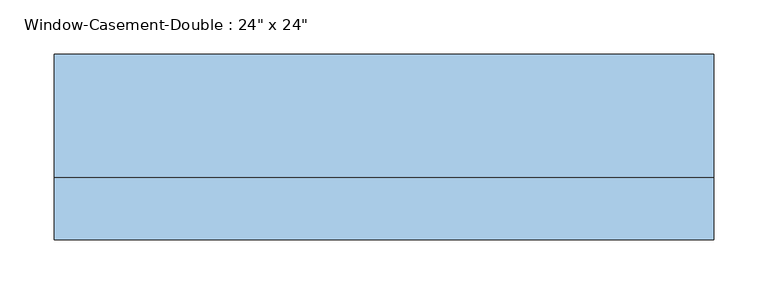
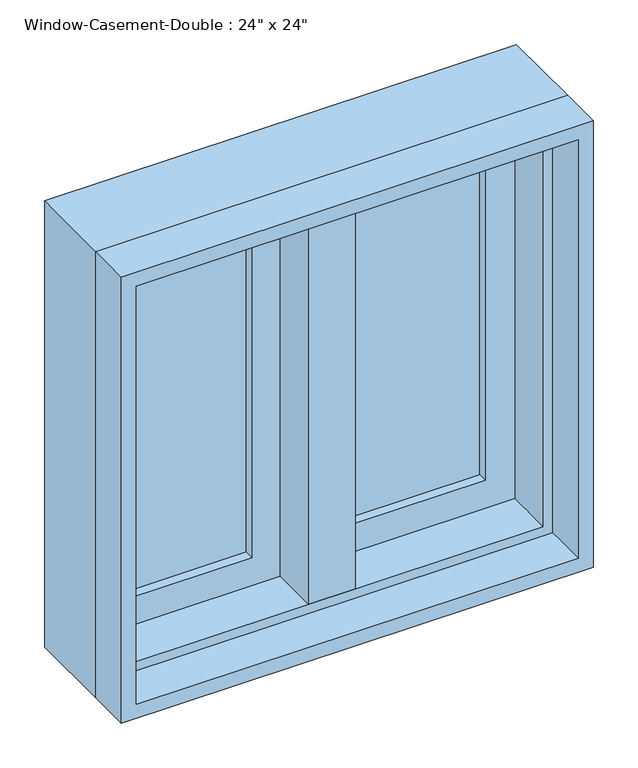
"""IFC4 building model written with IfcOpenShell, lengths in millimetres: window geometry."""

from ifc_helpers import new_model, si_unit, frame, origin, place, context, project, spatial, polyline, outline, extrude, faceted_brep, source, transform, mapped, element, save


def window_0c121b81(model_context):
    return source(origin(), model_context, "Body", "SolidModel", [
        faceted_brep([(9.525, 95.25, 1511.3), (-9.525, 95.25, 1511.3), (-9.525, 44.45, 1511.3), (9.525, 44.45, 1511.3), (9.525, 95.25, 927.1), (9.525, 44.45, 927.1), (-9.525, 44.45, 927.1), (-9.525, 95.25, 927.1), (-9.525, 44.45, 946.15), (-9.525, 44.45, 1492.25), (-30.1625, 44.45, 946.15), (-30.1625, 44.45, 1492.25), (-30.1625, -19.05, 946.15), (-30.1625, -19.05, 1492.25), (30.1625, -19.05, 946.15), (30.1625, -19.05, 1492.25), (30.1625, 44.45, 946.15), (30.1625, 44.45, 1492.25), (9.525, 44.45, 946.15), (9.525, 44.45, 1492.25)], [[[0, 1, 2, 3]], [[4, 5, 6, 7]], [[1, 0, 4, 7]], [[2, 1, 7, 6, 8, 9]], [[9, 8, 10, 11]], [[11, 10, 12, 13]], [[13, 12, 14, 15]], [[15, 14, 16, 17]], [[17, 16, 18, 19]], [[0, 3, 19, 18, 5, 4]], [[18, 8, 6, 5]], [[9, 19, 3, 2]], [[8, 18, 16, 14, 12, 10]], [[19, 9, 11, 13, 15, 17]]]),
        extrude(outline(polyline([(-66.675, 76.2), (-66.675, 69.85), (-234.95, 69.85), (-234.95, 76.2), (-66.675, 76.2)])), frame((0.0, 0.0, 984.25), z_axis=(0.0, 0.0, 1.0), x_axis=(1.0, 0.0, 0.0)), (0.0, 0.0, 1.0), 469.9),
        extrude(outline(polyline([(-234.95, 57.15), (-234.95, 63.5), (-66.675, 63.5), (-66.675, 57.15), (-234.95, 57.15)])), frame((0.0, 0.0, 984.25), z_axis=(0.0, 0.0, 1.0), x_axis=(1.0, 0.0, 0.0)), (0.0, 0.0, 1.0), 469.9),
        extrude(outline(polyline([(234.95, 76.2), (234.95, 69.85), (66.675, 69.85), (66.675, 76.2), (234.95, 76.2)])), frame((0.0, 0.0, 984.25), z_axis=(0.0, 0.0, 1.0), x_axis=(1.0, 0.0, 0.0)), (0.0, 0.0, 1.0), 469.9),
        extrude(outline(polyline([(66.675, 57.15), (66.675, 63.5), (234.95, 63.5), (234.95, 57.15), (66.675, 57.15)])), frame((0.0, 0.0, 984.25), z_axis=(0.0, 0.0, 1.0), x_axis=(1.0, 0.0, 0.0)), (0.0, 0.0, 1.0), 469.9),
        extrude(outline(polyline([(1511.3, -292.1), (927.1, -292.1), (927.1, -9.525), (1511.3, -9.525), (1511.3, -292.1)]), holes=[polyline([(1454.15, -66.675), (984.25, -66.675), (984.25, -234.95), (1454.15, -234.95), (1454.15, -66.675)])]), frame((0.0, 44.45, 0.0), z_axis=(0.0, 1.0, 0.0), x_axis=(0.0, 0.0, 1.0)), (0.0, 0.0, 1.0), 44.45),
        extrude(outline(polyline([(927.1, 292.1), (1511.3, 292.1), (1511.3, 9.525), (927.1, 9.525), (927.1, 292.1)]), holes=[polyline([(984.25, 66.675), (1454.15, 66.675), (1454.15, 234.95), (984.25, 234.95), (984.25, 66.675)])]), frame((0.0, 44.45, 0.0), z_axis=(0.0, 1.0, 0.0), x_axis=(0.0, 0.0, 1.0)), (0.0, 0.0, 1.0), 44.45),
        extrude(outline(polyline([(1524.0, -304.8), (914.4, -304.8), (914.4, 304.8), (1524.0, 304.8), (1524.0, -304.8)]), holes=[polyline([(1504.95, 285.75), (933.45, 285.75), (933.45, -285.75), (1504.95, -285.75), (1504.95, 285.75)])]), frame((0.0, -76.2, 0.0), z_axis=(0.0, 1.0, 0.0), x_axis=(0.0, 0.0, 1.0)), (0.0, 0.0, 1.0), 57.15),
        faceted_brep([(273.05, 44.45, 1492.25), (273.05, -19.05, 1492.25), (-273.05, -19.05, 1492.25), (-273.05, 44.45, 1492.25), (292.1, 95.25, 1511.3), (292.1, 44.45, 1511.3), (-292.1, 44.45, 1511.3), (-292.1, 95.25, 1511.3), (304.8, -19.05, 1524.0), (304.8, 95.25, 1524.0), (-304.8, 95.25, 1524.0), (-304.8, -19.05, 1524.0), (-273.05, -19.05, 946.15), (-273.05, 44.45, 946.15), (-292.1, 44.45, 927.1), (-292.1, 95.25, 927.1), (-304.8, 95.25, 914.4), (-304.8, -19.05, 914.4), (273.05, -19.05, 946.15), (273.05, 44.45, 946.15), (292.1, 44.45, 927.1), (292.1, 95.25, 927.1), (304.8, 95.25, 914.4), (304.8, -19.05, 914.4)], [[[0, 1, 2, 3]], [[4, 5, 6, 7]], [[8, 9, 10, 11]], [[3, 2, 12, 13]], [[7, 6, 14, 15]], [[11, 10, 16, 17]], [[13, 12, 18, 19]], [[15, 14, 20, 21]], [[17, 16, 22, 23]], [[11, 17, 23, 8], [1, 18, 12, 2]], [[19, 18, 1, 0]], [[5, 20, 14, 6], [3, 13, 19, 0]], [[21, 20, 5, 4]], [[23, 22, 9, 8]], [[9, 22, 16, 10], [7, 15, 21, 4]]]),
    ])


if __name__ == "__main__":
    model = new_model("IFC4")
    model_context = context("Model", 3, world=origin())
    ifc_project = project(units=[si_unit("LENGTHUNIT", "METRE", prefix="MILLI")], contexts=[model_context])
    site = spatial("IfcSite", under=ifc_project)
    building = spatial("IfcBuilding", under=site)
    placement = place(None, origin())
    window_shape = window_0c121b81(model_context)
    element("IfcWindow", 1, ObjectType="Window-Casement-Double : 24\" x 24\"", at=placement, inside=building, context=model_context, shape_type="MappedRepresentation", body=[
        mapped(window_shape, transform((0.0, 0.0, 0.0), x_axis=(1.0, 0.0, 0.0), y_axis=(0.0, 1.0, 0.0), z_axis=(0.0, 0.0, 1.0))),
    ])
    save(model, "model.ifc")

# Revit data of these elements
# Type "Window-Casement-Double : 24\" x 24\""
#   Type Mark = "14"
#   Fire Rating = "0.5h"
#   Assembly Code = "B2020100"
#   Analytic Construction = "Double glazing - domestic"
#   Frame Extension [instance default] = 0' - 0 1/4"
#   Window Inset [instance default] = 0' - 0"
#   Wall Thickness [instance default] = 0' - 6"
#   Interior Wall Closure [instance default] = 0' - 2 1/4"
#   Half Width = 1' - 0"
#   Visual Light Transmittance = 0.81
#   Thermal Resistance (R) = 1.8146 (h·ft²·°F)/BTU
#   Solar Heat Gain Coefficient = 0.76
#   Rough Width = 2' - 0 1/2"
#   Rough Height = 2' - 0 1/2"
#   Height = 2' - 0"
#   Heat Transfer Coefficient (U) = 0.5511 BTU/(h·ft²·°F)
#   Exterior Wall Closure [instance default] = 0' - 1 1/4"
#   Extension Jamb [instance default] = 0' - 2 1/4"
#   Default Sill Height = 3' - 0"
#   Width = 2' - 0"
#   Define Thermal Properties by = 0
#   Muntin Visibility = yes
#   Interior Trim Visibility [instance default] = yes
#   Exterior Trim Visibility [instance default] = yes
#   Extension Jamb Visibility [instance default] = yes
#   Interior Trim Material = Wood - Stained
#   Muntin Pattern = Muntin Pattern_2x2 : Muntin Pattern_2x2
#   Interior Trim = Trim-Window-Interior-Flat : Picture Frame
#   Interior Frame Material = Wood - Stained
#   Glass Panel Material = Glass
#   Exterior Trim Material = Clad - White
#   Exterior Trim = Trim-Window-Exterior-Flat : with Sill
#   Exterior Frame Material = Clad - White
#   Wall Closure = (empty or 0)
# Element 1 (IfcWindow, "Window-Casement-Double : 24\" x 24\"")
#   Materials on its faces: "Wood - Stained", "Glass", "Clad - White"
# Materials
#   "Wood - Stained": class "Wood", colour RGB 224 178 126, transparency 0, Cost = 0
#   "Glass": class "Glass", colour RGB 0 128 192, transparency 0.75, Description = "Soda Lime Glass", Cost = 0
#   "Clad - White": class "Wood", colour RGB 242 242 238, transparency 0, Cost = 0
